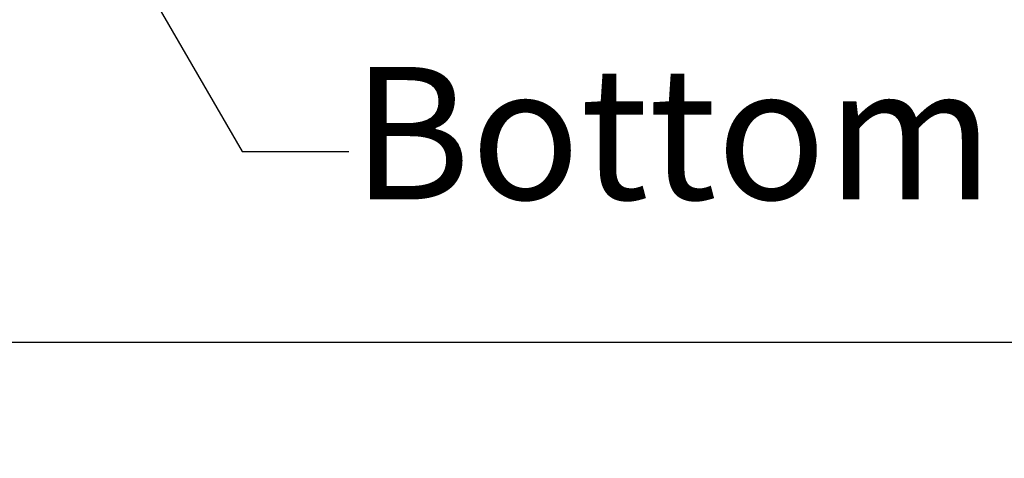
# Model space of a CAD drawing. Units: inches. Extents: x -12 to 334, y -10 to 186.
# Tile 48 of 77: x 227 to 257, y 11 to 24. Entities that reach past the tile are written whole.
import ezdxf
from ezdxf import colors
from ezdxf.entities.mleader import LeaderData, LeaderLine
from ezdxf.math import Vec2, Vec3

# ---------------------------------------------------------------- set-up
doc = ezdxf.new("R2010")
doc.units = ezdxf.units.IN
doc.header["$MEASUREMENT"] = 0
doc.layers.add('M-ANNO-TEXT', color=3, linetype='Continuous', lineweight=25)
doc.layers.add('M-DIMS', color=2, linetype='Continuous', lineweight=18)
doc.styles.get("Standard").update_dxf_attribs({"font": 'arial.ttf'})
doc.dimstyles.get("Standard").update_dxf_attribs({"dimtxt": 0.18, "dimasz": 0.18, "dimexe": 0.18, "dimexo": 0.0625, "dimgap": 0.09, "dimtad": 0, "dimtih": 1, "dimtoh": 1, "dimdec": 4, "dimzin": 0, "dimdsep": 46, "dimtxsty": 'Standard', "dimcen": 0.09, "dimadec": 0, "dimazin": 0, "dimtfac": 1, "dimtdec": 4, "dimtofl": 0, "dimtmove": 0, "dimatfit": 3, "dimfxl": 1, "dimtolj": 1, "dimtzin": 0, "dimarcsym": 0})

# ---------------------------------------------------------------- blocks, each defined once
blk = doc.blocks.new('*D1')
at = {"layer": 'Defpoints', "color": 0, "transparency": 16777216}
for p in [(281.426, 91.899), (3.376, 80.692), (281.426, 14.304)]:
    blk.add_point(p, dxfattribs=at)
at = {"layer": 'M-DIMS', "color": 0, "lineweight": -2, "transparency": 16777216}
for p, q in [((281.426, 91.836), (281.426, 14.124)), ((3.376, 80.629), (3.376, 14.124)), ((3.556, 14.304), (141.935, 14.304)), ((281.246, 14.304), (142.867, 14.304))]:
    blk.add_line(p, q, dxfattribs=at)
at = {"layer": 'M-DIMS', "color": 0, "transparency": 16777216}
for points in [[(3.556, 14.334), (3.556, 14.274), (3.376, 14.304)], [(281.246, 14.334), (281.246, 14.274), (281.426, 14.304)]]:
    blk.add_solid(points, dxfattribs=at)
at = {"layer": 'M-DIMS', "color": 0, "transparency": 16777216, "insert": (142.401, 14.304), "char_height": 0.18, "attachment_point": 5}
blk.add_mtext('\\A1;278.05', dxfattribs=at)

msp = doc.modelspace()

# ---------------------------------------------------------------- dimensions: what is measured, and where the dimension line sits
at = {"layer": 'M-DIMS'}
dim = msp.add_linear_dim(base=(281.4256, 14.3041), p1=(3.3765, 80.6915), p2=(281.4256, 91.8988), dimstyle='Standard', override={"dimdec": 2, "dimlfac": 1, "dimrnd": 0, "dimzin": 0, "dimdsep": 46, "dimlunit": 2}, dxfattribs=at)
dim.commit()
dim.dimension.update_dxf_attribs({"geometry": '*D1', "text_midpoint": (142.401, 14.3041)})

# ---------------------------------------------------------------- leaders
at = {"layer": 'M-ANNO-TEXT'}
ml = msp.add_multileader_mtext('Standard', dxfattribs=at)
ml.set_content('Bottom product', color=256)
ml.set_leader_properties()
ml.build(insert=Vec2(0, 0))
ml.multileader.update_dxf_attribs({"dogleg_length": 0.36, "arrow_head_size": 0.7})
ctx = ml.context
ctx.base_point, ctx.arrow_head_size, ctx.landing_gap_size, ctx.plane_origin = Vec3(237.0261, 20.0676), 0.7, 0.09, Vec3(227.5761, 30.8541)
notes = []
notes.append((ctx, [(0, (1, 1, 0), (233.8037, 20.0676), (1, 0), 3.2224, [(0, [(227.5761, 30.8541)], 0, [])])]))
ctx.mtext.insert, ctx.mtext.flow_direction = Vec3(237.1161, 22.6228), 5
for ctx, leaders in notes:
    for number, flags, end, landing, length, lines in leaders:
        leader = LeaderData()
        leader.index, (leader.has_last_leader_line, leader.has_dogleg_vector, leader.attachment_direction) = number, flags
        leader.last_leader_point, leader.dogleg_vector, leader.dogleg_length = Vec3(end), Vec3(landing), length
        for number, points, colour, breaks in lines:
            line = LeaderLine()
            line.index, line.vertices, line.color, line.breaks = number, Vec3.list(points), colors.encode_raw_color(colour), breaks
            leader.lines.append(line)
        ctx.leaders.append(leader)

doc.saveas('drawing.dxf')
